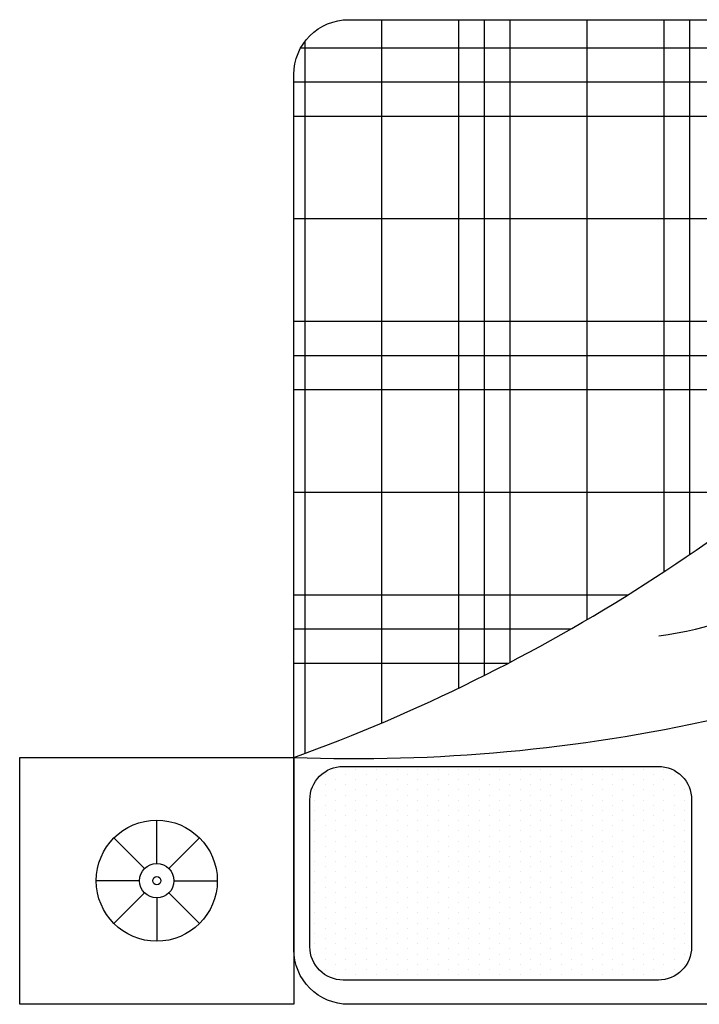
# Model space of a CAD drawing. Units: millimetres. Extents: x 2817 to 5038, y 1110 to 3565.
# Tile 20 of 21: x 4946 to 4992, y 3499 to 3565. Entities that reach past the tile are written whole.
import ezdxf

# ---------------------------------------------------------------- set-up
doc = ezdxf.new("R2010")
doc.units = ezdxf.units.MM
doc.layers.add('BLOCK', color=6, linetype='Continuous')
doc.layers.add('FURNITURE', color=219, linetype='Continuous', lineweight=18)

# ---------------------------------------------------------------- blocks, each defined once
blk = doc.blocks.new('*X7')
at = {"color": 0}
for p, q in [((276.598, 451.25), (280.51, 451.25)), ((275.455, 450.625), (280.51, 450.625)), ((274.411, 450), (280.51, 450)), ((265.51, 448.125), (267.634, 448.125)), ((271.723, 448.125), (280.51, 448.125)), ((265.51, 446.25), (268.465, 446.25)), ((269.519, 446.25), (280.51, 446.25)), ((265.51, 445.625), (268.531, 445.625)), ((268.866, 445.625), (280.51, 445.625)), ((265.51, 445), (280.51, 445)), ((265.51, 443.125), (280.51, 443.125)), ((265.51, 441.25), (280.51, 441.25)), ((265.51, 440.625), (280.51, 440.625)), ((265.634, 440), (280.386, 440))]:
    blk.add_line(p, q, dxfattribs=at)
blk = doc.blocks.new('*X8')
at = {"color": 0}
for p, q in [((280.312, 439.886), (280.312, 452.896)), ((278.906, 439.482), (278.906, 452.338)), ((277.5, 439.482), (277.5, 451.702)), ((277.031, 439.482), (277.031, 451.471)), ((276.562, 439.482), (276.562, 451.231)), ((275.156, 439.482), (275.156, 450.451)), ((265.781, 439.797), (265.781, 449.511)), ((273.75, 439.482), (273.75, 449.576)), ((266.25, 439.517), (266.25, 449.296)), ((273.281, 439.482), (273.281, 449.261)), ((272.812, 439.482), (272.812, 448.934)), ((267.656, 439.482), (267.656, 448.095)), ((271.406, 439.482), (271.406, 447.876)), ((270, 439.482), (270, 446.689)), ((269.531, 439.482), (269.531, 446.262)), ((269.062, 439.482), (269.062, 445.817))]:
    blk.add_line(p, q, dxfattribs=at)
blk = doc.blocks.new('*X9')
at = {"color": 0}
for p, q in [((273.9375, 457.03125), (273.9375, 457.03125)), ((274.3125, 457.03125), (274.3125, 457.03125)), ((274.6875, 457.03125), (274.6875, 457.03125)), ((275.0625, 457.03125), (275.0625, 457.03125)), ((275.4375, 457.03125), (275.4375, 457.03125)), ((275.8125, 457.03125), (275.8125, 457.03125)), ((276.1875, 457.03125), (276.1875, 457.03125)), ((276.5625, 457.03125), (276.5625, 457.03125)), ((276.9375, 457.03125), (276.9375, 457.03125)), ((277.3125, 457.03125), (277.3125, 457.03125)), ((277.6875, 457.03125), (277.6875, 457.03125)), ((278.0625, 457.03125), (278.0625, 457.03125)), ((278.4375, 457.03125), (278.4375, 457.03125)), ((278.8125, 457.03125), (278.8125, 457.03125)), ((279.1875, 457.03125), (279.1875, 457.03125)), ((279.5625, 457.03125), (279.5625, 457.03125)), ((273.5625, 456.84375), (273.5625, 456.84375)), ((273.75, 456.9375), (273.75, 456.9375)), ((273.9375, 456.84375), (273.9375, 456.84375)), ((274.125, 456.9375), (274.125, 456.9375)), ((274.3125, 456.84375), (274.3125, 456.84375)), ((274.5, 456.9375), (274.5, 456.9375)), ((274.6875, 456.84375), (274.6875, 456.84375)), ((274.875, 456.9375), (274.875, 456.9375)), ((275.0625, 456.84375), (275.0625, 456.84375)), ((275.25, 456.9375), (275.25, 456.9375)), ((275.4375, 456.84375), (275.4375, 456.84375)), ((275.625, 456.9375), (275.625, 456.9375)), ((275.8125, 456.84375), (275.8125, 456.84375)), ((276, 456.9375), (276, 456.9375)), ((276.1875, 456.84375), (276.1875, 456.84375)), ((276.375, 456.9375), (276.375, 456.9375)), ((276.5625, 456.84375), (276.5625, 456.84375)), ((276.75, 456.9375), (276.75, 456.9375)), ((276.9375, 456.84375), (276.9375, 456.84375)), ((277.125, 456.9375), (277.125, 456.9375)), ((277.3125, 456.84375), (277.3125, 456.84375)), ((277.5, 456.9375), (277.5, 456.9375)), ((277.6875, 456.84375), (277.6875, 456.84375)), ((277.875, 456.9375), (277.875, 456.9375)), ((278.0625, 456.84375), (278.0625, 456.84375)), ((278.25, 456.9375), (278.25, 456.9375)), ((278.4375, 456.84375), (278.4375, 456.84375)), ((278.625, 456.9375), (278.625, 456.9375)), ((278.8125, 456.84375), (278.8125, 456.84375)), ((279, 456.9375), (279, 456.9375)), ((279.1875, 456.84375), (279.1875, 456.84375)), ((279.375, 456.9375), (279.375, 456.9375)), ((279.5625, 456.84375), (279.5625, 456.84375)), ((279.75, 456.9375), (279.75, 456.9375)), ((279.9375, 456.84375), (279.9375, 456.84375)), ((273.375, 456.75), (273.375, 456.75)), ((273.75, 456.75), (273.75, 456.75)), ((274.125, 456.75), (274.125, 456.75)), ((274.5, 456.75), (274.5, 456.75)), ((274.875, 456.75), (274.875, 456.75)), ((275.25, 456.75), (275.25, 456.75)), ((275.625, 456.75), (275.625, 456.75)), ((276, 456.75), (276, 456.75)), ((276.375, 456.75), (276.375, 456.75)), ((276.75, 456.75), (276.75, 456.75)), ((277.125, 456.75), (277.125, 456.75)), ((277.5, 456.75), (277.5, 456.75)), ((277.875, 456.75), (277.875, 456.75)), ((278.25, 456.75), (278.25, 456.75)), ((278.625, 456.75), (278.625, 456.75)), ((279, 456.75), (279, 456.75)), ((279.375, 456.75), (279.375, 456.75)), ((279.75, 456.75), (279.75, 456.75)), ((280.125, 456.75), (280.125, 456.75)), ((273.375, 456.5625), (273.375, 456.5625)), ((273.5625, 456.65625), (273.5625, 456.65625)), ((273.75, 456.5625), (273.75, 456.5625)), ((273.9375, 456.65625), (273.9375, 456.65625)), ((274.125, 456.5625), (274.125, 456.5625)), ((274.3125, 456.65625), (274.3125, 456.65625)), ((274.5, 456.5625), (274.5, 456.5625)), ((274.6875, 456.65625), (274.6875, 456.65625)), ((274.875, 456.5625), (274.875, 456.5625)), ((275.0625, 456.65625), (275.0625, 456.65625)), ((275.25, 456.5625), (275.25, 456.5625)), ((275.4375, 456.65625), (275.4375, 456.65625)), ((275.625, 456.5625), (275.625, 456.5625)), ((275.8125, 456.65625), (275.8125, 456.65625)), ((276, 456.5625), (276, 456.5625)), ((276.1875, 456.65625), (276.1875, 456.65625)), ((276.375, 456.5625), (276.375, 456.5625)), ((276.5625, 456.65625), (276.5625, 456.65625)), ((276.75, 456.5625), (276.75, 456.5625)), ((276.9375, 456.65625), (276.9375, 456.65625)), ((277.125, 456.5625), (277.125, 456.5625)), ((277.3125, 456.65625), (277.3125, 456.65625)), ((277.5, 456.5625), (277.5, 456.5625)), ((277.6875, 456.65625), (277.6875, 456.65625)), ((277.875, 456.5625), (277.875, 456.5625)), ((278.0625, 456.65625), (278.0625, 456.65625)), ((278.25, 456.5625), (278.25, 456.5625)), ((278.4375, 456.65625), (278.4375, 456.65625)), ((278.625, 456.5625), (278.625, 456.5625)), ((278.8125, 456.65625), (278.8125, 456.65625)), ((279, 456.5625), (279, 456.5625)), ((279.1875, 456.65625), (279.1875, 456.65625)), ((279.375, 456.5625), (279.375, 456.5625)), ((279.5625, 456.65625), (279.5625, 456.65625)), ((279.75, 456.5625), (279.75, 456.5625)), ((279.9375, 456.65625), (279.9375, 456.65625)), ((280.125, 456.5625), (280.125, 456.5625)), ((273.375, 456.375), (273.375, 456.375)), ((273.5625, 456.46875), (273.5625, 456.46875)), ((273.75, 456.375), (273.75, 456.375)), ((273.9375, 456.46875), (273.9375, 456.46875)), ((274.125, 456.375), (274.125, 456.375)), ((274.3125, 456.46875), (274.3125, 456.46875)), ((274.5, 456.375), (274.5, 456.375)), ((274.6875, 456.46875), (274.6875, 456.46875)), ((274.875, 456.375), (274.875, 456.375)), ((275.0625, 456.46875), (275.0625, 456.46875)), ((275.25, 456.375), (275.25, 456.375)), ((275.4375, 456.46875), (275.4375, 456.46875)), ((275.625, 456.375), (275.625, 456.375)), ((275.8125, 456.46875), (275.8125, 456.46875)), ((276, 456.375), (276, 456.375)), ((276.1875, 456.46875), (276.1875, 456.46875)), ((276.375, 456.375), (276.375, 456.375)), ((276.5625, 456.46875), (276.5625, 456.46875)), ((276.75, 456.375), (276.75, 456.375)), ((276.9375, 456.46875), (276.9375, 456.46875)), ((277.125, 456.375), (277.125, 456.375)), ((277.3125, 456.46875), (277.3125, 456.46875)), ((277.5, 456.375), (277.5, 456.375)), ((277.6875, 456.46875), (277.6875, 456.46875)), ((277.875, 456.375), (277.875, 456.375)), ((278.0625, 456.46875), (278.0625, 456.46875)), ((278.25, 456.375), (278.25, 456.375)), ((278.4375, 456.46875), (278.4375, 456.46875)), ((278.625, 456.375), (278.625, 456.375)), ((278.8125, 456.46875), (278.8125, 456.46875)), ((279, 456.375), (279, 456.375)), ((279.1875, 456.46875), (279.1875, 456.46875)), ((279.375, 456.375), (279.375, 456.375)), ((279.5625, 456.46875), (279.5625, 456.46875)), ((279.75, 456.375), (279.75, 456.375)), ((279.9375, 456.46875), (279.9375, 456.46875)), ((280.125, 456.375), (280.125, 456.375)), ((273.375, 456.1875), (273.375, 456.1875)), ((273.5625, 456.28125), (273.5625, 456.28125)), ((273.75, 456.1875), (273.75, 456.1875)), ((273.9375, 456.28125), (273.9375, 456.28125)), ((274.125, 456.1875), (274.125, 456.1875)), ((274.3125, 456.28125), (274.3125, 456.28125)), ((274.5, 456.1875), (274.5, 456.1875)), ((274.6875, 456.28125), (274.6875, 456.28125)), ((274.875, 456.1875), (274.875, 456.1875)), ((275.0625, 456.28125), (275.0625, 456.28125)), ((275.25, 456.1875), (275.25, 456.1875)), ((275.4375, 456.28125), (275.4375, 456.28125)), ((275.625, 456.1875), (275.625, 456.1875)), ((275.8125, 456.28125), (275.8125, 456.28125)), ((276, 456.1875), (276, 456.1875)), ((276.1875, 456.28125), (276.1875, 456.28125)), ((276.375, 456.1875), (276.375, 456.1875)), ((276.5625, 456.28125), (276.5625, 456.28125)), ((276.75, 456.1875), (276.75, 456.1875)), ((276.9375, 456.28125), (276.9375, 456.28125)), ((277.125, 456.1875), (277.125, 456.1875)), ((277.3125, 456.28125), (277.3125, 456.28125)), ((277.5, 456.1875), (277.5, 456.1875)), ((277.6875, 456.28125), (277.6875, 456.28125)), ((277.875, 456.1875), (277.875, 456.1875)), ((278.0625, 456.28125), (278.0625, 456.28125)), ((278.25, 456.1875), (278.25, 456.1875)), ((278.4375, 456.28125), (278.4375, 456.28125)), ((278.625, 456.1875), (278.625, 456.1875)), ((278.8125, 456.28125), (278.8125, 456.28125)), ((279, 456.1875), (279, 456.1875)), ((279.1875, 456.28125), (279.1875, 456.28125)), ((279.375, 456.1875), (279.375, 456.1875)), ((279.5625, 456.28125), (279.5625, 456.28125)), ((279.75, 456.1875), (279.75, 456.1875)), ((279.9375, 456.28125), (279.9375, 456.28125)), ((280.125, 456.1875), (280.125, 456.1875)), ((273.375, 456), (273.375, 456)), ((273.5625, 456.09375), (273.5625, 456.09375)), ((273.75, 456), (273.75, 456)), ((273.9375, 456.09375), (273.9375, 456.09375)), ((274.125, 456), (274.125, 456)), ((274.3125, 456.09375), (274.3125, 456.09375)), ((274.5, 456), (274.5, 456)), ((274.6875, 456.09375), (274.6875, 456.09375)), ((274.875, 456), (274.875, 456)), ((275.0625, 456.09375), (275.0625, 456.09375)), ((275.25, 456), (275.25, 456)), ((275.4375, 456.09375), (275.4375, 456.09375)), ((275.625, 456), (275.625, 456)), ((275.8125, 456.09375), (275.8125, 456.09375)), ((276, 456), (276, 456)), ((276.1875, 456.09375), (276.1875, 456.09375)), ((276.375, 456), (276.375, 456)), ((276.5625, 456.09375), (276.5625, 456.09375)), ((276.75, 456), (276.75, 456)), ((276.9375, 456.09375), (276.9375, 456.09375)), ((277.125, 456), (277.125, 456)), ((277.3125, 456.09375), (277.3125, 456.09375)), ((277.5, 456), (277.5, 456)), ((277.6875, 456.09375), (277.6875, 456.09375)), ((277.875, 456), (277.875, 456)), ((278.0625, 456.09375), (278.0625, 456.09375)), ((278.25, 456), (278.25, 456)), ((278.4375, 456.09375), (278.4375, 456.09375)), ((278.625, 456), (278.625, 456)), ((278.8125, 456.09375), (278.8125, 456.09375)), ((279, 456), (279, 456)), ((279.1875, 456.09375), (279.1875, 456.09375)), ((279.375, 456), (279.375, 456)), ((279.5625, 456.09375), (279.5625, 456.09375)), ((279.75, 456), (279.75, 456)), ((279.9375, 456.09375), (279.9375, 456.09375)), ((280.125, 456), (280.125, 456)), ((273.375, 455.8125), (273.375, 455.8125)), ((273.5625, 455.90625), (273.5625, 455.90625)), ((273.75, 455.8125), (273.75, 455.8125)), ((273.9375, 455.90625), (273.9375, 455.90625)), ((274.125, 455.8125), (274.125, 455.8125)), ((274.3125, 455.90625), (274.3125, 455.90625)), ((274.5, 455.8125), (274.5, 455.8125)), ((274.6875, 455.90625), (274.6875, 455.90625)), ((274.875, 455.8125), (274.875, 455.8125)), ((275.0625, 455.90625), (275.0625, 455.90625)), ((275.25, 455.8125), (275.25, 455.8125)), ((275.4375, 455.90625), (275.4375, 455.90625)), ((275.625, 455.8125), (275.625, 455.8125)), ((275.8125, 455.90625), (275.8125, 455.90625)), ((276, 455.8125), (276, 455.8125)), ((276.1875, 455.90625), (276.1875, 455.90625)), ((276.375, 455.8125), (276.375, 455.8125)), ((276.5625, 455.90625), (276.5625, 455.90625)), ((276.75, 455.8125), (276.75, 455.8125)), ((276.9375, 455.90625), (276.9375, 455.90625)), ((277.125, 455.8125), (277.125, 455.8125)), ((277.3125, 455.90625), (277.3125, 455.90625)), ((277.5, 455.8125), (277.5, 455.8125)), ((277.6875, 455.90625), (277.6875, 455.90625)), ((277.875, 455.8125), (277.875, 455.8125)), ((278.0625, 455.90625), (278.0625, 455.90625)), ((278.25, 455.8125), (278.25, 455.8125)), ((278.4375, 455.90625), (278.4375, 455.90625)), ((278.625, 455.8125), (278.625, 455.8125)), ((278.8125, 455.90625), (278.8125, 455.90625)), ((279, 455.8125), (279, 455.8125)), ((279.1875, 455.90625), (279.1875, 455.90625)), ((279.375, 455.8125), (279.375, 455.8125)), ((279.5625, 455.90625), (279.5625, 455.90625)), ((279.75, 455.8125), (279.75, 455.8125)), ((279.9375, 455.90625), (279.9375, 455.90625)), ((280.125, 455.8125), (280.125, 455.8125)), ((273.375, 455.625), (273.375, 455.625)), ((273.5625, 455.71875), (273.5625, 455.71875)), ((273.75, 455.625), (273.75, 455.625)), ((273.9375, 455.71875), (273.9375, 455.71875)), ((274.125, 455.625), (274.125, 455.625)), ((274.3125, 455.71875), (274.3125, 455.71875)), ((274.5, 455.625), (274.5, 455.625)), ((274.6875, 455.71875), (274.6875, 455.71875)), ((274.875, 455.625), (274.875, 455.625)), ((275.0625, 455.71875), (275.0625, 455.71875)), ((275.25, 455.625), (275.25, 455.625)), ((275.4375, 455.71875), (275.4375, 455.71875)), ((275.625, 455.625), (275.625, 455.625)), ((275.8125, 455.71875), (275.8125, 455.71875)), ((276, 455.625), (276, 455.625)), ((276.1875, 455.71875), (276.1875, 455.71875)), ((276.375, 455.625), (276.375, 455.625)), ((276.5625, 455.71875), (276.5625, 455.71875)), ((276.75, 455.625), (276.75, 455.625)), ((276.9375, 455.71875), (276.9375, 455.71875)), ((277.125, 455.625), (277.125, 455.625)), ((277.3125, 455.71875), (277.3125, 455.71875)), ((277.5, 455.625), (277.5, 455.625)), ((277.6875, 455.71875), (277.6875, 455.71875)), ((277.875, 455.625), (277.875, 455.625)), ((278.0625, 455.71875), (278.0625, 455.71875)), ((278.25, 455.625), (278.25, 455.625)), ((278.4375, 455.71875), (278.4375, 455.71875)), ((278.625, 455.625), (278.625, 455.625)), ((278.8125, 455.71875), (278.8125, 455.71875)), ((279, 455.625), (279, 455.625)), ((279.1875, 455.71875), (279.1875, 455.71875)), ((279.375, 455.625), (279.375, 455.625)), ((279.5625, 455.71875), (279.5625, 455.71875)), ((279.75, 455.625), (279.75, 455.625)), ((279.9375, 455.71875), (279.9375, 455.71875)), ((280.125, 455.625), (280.125, 455.625)), ((273.375, 455.4375), (273.375, 455.4375)), ((273.5625, 455.53125), (273.5625, 455.53125)), ((273.75, 455.4375), (273.75, 455.4375)), ((273.9375, 455.53125), (273.9375, 455.53125)), ((274.125, 455.4375), (274.125, 455.4375)), ((274.3125, 455.53125), (274.3125, 455.53125)), ((274.5, 455.4375), (274.5, 455.4375)), ((274.6875, 455.53125), (274.6875, 455.53125)), ((274.875, 455.4375), (274.875, 455.4375)), ((275.0625, 455.53125), (275.0625, 455.53125)), ((275.25, 455.4375), (275.25, 455.4375)), ((275.4375, 455.53125), (275.4375, 455.53125)), ((275.625, 455.4375), (275.625, 455.4375)), ((275.8125, 455.53125), (275.8125, 455.53125)), ((276, 455.4375), (276, 455.4375)), ((276.1875, 455.53125), (276.1875, 455.53125)), ((276.375, 455.4375), (276.375, 455.4375)), ((276.5625, 455.53125), (276.5625, 455.53125)), ((276.75, 455.4375), (276.75, 455.4375)), ((276.9375, 455.53125), (276.9375, 455.53125)), ((277.125, 455.4375), (277.125, 455.4375)), ((277.3125, 455.53125), (277.3125, 455.53125)), ((277.5, 455.4375), (277.5, 455.4375)), ((277.6875, 455.53125), (277.6875, 455.53125)), ((277.875, 455.4375), (277.875, 455.4375)), ((278.0625, 455.53125), (278.0625, 455.53125)), ((278.25, 455.4375), (278.25, 455.4375)), ((278.4375, 455.53125), (278.4375, 455.53125)), ((278.625, 455.4375), (278.625, 455.4375)), ((278.8125, 455.53125), (278.8125, 455.53125)), ((279, 455.4375), (279, 455.4375)), ((279.1875, 455.53125), (279.1875, 455.53125)), ((279.375, 455.4375), (279.375, 455.4375)), ((279.5625, 455.53125), (279.5625, 455.53125)), ((279.75, 455.4375), (279.75, 455.4375)), ((279.9375, 455.53125), (279.9375, 455.53125)), ((280.125, 455.4375), (280.125, 455.4375)), ((273.375, 455.25), (273.375, 455.25)), ((273.5625, 455.34375), (273.5625, 455.34375)), ((273.75, 455.25), (273.75, 455.25)), ((273.9375, 455.34375), (273.9375, 455.34375)), ((274.125, 455.25), (274.125, 455.25)), ((274.3125, 455.34375), (274.3125, 455.34375)), ((274.5, 455.25), (274.5, 455.25)), ((274.6875, 455.34375), (274.6875, 455.34375)), ((274.875, 455.25), (274.875, 455.25)), ((275.0625, 455.34375), (275.0625, 455.34375)), ((275.25, 455.25), (275.25, 455.25)), ((275.4375, 455.34375), (275.4375, 455.34375)), ((275.625, 455.25), (275.625, 455.25)), ((275.8125, 455.34375), (275.8125, 455.34375)), ((276, 455.25), (276, 455.25)), ((276.1875, 455.34375), (276.1875, 455.34375)), ((276.375, 455.25), (276.375, 455.25)), ((276.5625, 455.34375), (276.5625, 455.34375)), ((276.75, 455.25), (276.75, 455.25)), ((276.9375, 455.34375), (276.9375, 455.34375)), ((277.125, 455.25), (277.125, 455.25)), ((277.3125, 455.34375), (277.3125, 455.34375)), ((277.5, 455.25), (277.5, 455.25)), ((277.6875, 455.34375), (277.6875, 455.34375)), ((277.875, 455.25), (277.875, 455.25)), ((278.0625, 455.34375), (278.0625, 455.34375)), ((278.25, 455.25), (278.25, 455.25)), ((278.4375, 455.34375), (278.4375, 455.34375)), ((278.625, 455.25), (278.625, 455.25)), ((278.8125, 455.34375), (278.8125, 455.34375)), ((279, 455.25), (279, 455.25)), ((279.1875, 455.34375), (279.1875, 455.34375)), ((279.375, 455.25), (279.375, 455.25)), ((279.5625, 455.34375), (279.5625, 455.34375)), ((279.75, 455.25), (279.75, 455.25)), ((279.9375, 455.34375), (279.9375, 455.34375)), ((280.125, 455.25), (280.125, 455.25)), ((273.375, 455.0625), (273.375, 455.0625)), ((273.5625, 455.15625), (273.5625, 455.15625)), ((273.75, 455.0625), (273.75, 455.0625)), ((273.9375, 455.15625), (273.9375, 455.15625)), ((274.125, 455.0625), (274.125, 455.0625)), ((274.3125, 455.15625), (274.3125, 455.15625)), ((274.5, 455.0625), (274.5, 455.0625)), ((274.6875, 455.15625), (274.6875, 455.15625)), ((274.875, 455.0625), (274.875, 455.0625)), ((275.0625, 455.15625), (275.0625, 455.15625)), ((275.25, 455.0625), (275.25, 455.0625)), ((275.4375, 455.15625), (275.4375, 455.15625)), ((275.625, 455.0625), (275.625, 455.0625)), ((275.8125, 455.15625), (275.8125, 455.15625)), ((276, 455.0625), (276, 455.0625)), ((276.1875, 455.15625), (276.1875, 455.15625)), ((276.375, 455.0625), (276.375, 455.0625)), ((276.5625, 455.15625), (276.5625, 455.15625)), ((276.75, 455.0625), (276.75, 455.0625)), ((276.9375, 455.15625), (276.9375, 455.15625)), ((277.125, 455.0625), (277.125, 455.0625)), ((277.3125, 455.15625), (277.3125, 455.15625)), ((277.5, 455.0625), (277.5, 455.0625)), ((277.6875, 455.15625), (277.6875, 455.15625)), ((277.875, 455.0625), (277.875, 455.0625)), ((278.0625, 455.15625), (278.0625, 455.15625)), ((278.25, 455.0625), (278.25, 455.0625)), ((278.4375, 455.15625), (278.4375, 455.15625)), ((278.625, 455.0625), (278.625, 455.0625)), ((278.8125, 455.15625), (278.8125, 455.15625)), ((279, 455.0625), (279, 455.0625)), ((279.1875, 455.15625), (279.1875, 455.15625)), ((279.375, 455.0625), (279.375, 455.0625)), ((279.5625, 455.15625), (279.5625, 455.15625)), ((279.75, 455.0625), (279.75, 455.0625)), ((279.9375, 455.15625), (279.9375, 455.15625)), ((280.125, 455.0625), (280.125, 455.0625)), ((273.375, 454.875), (273.375, 454.875)), ((273.5625, 454.96875), (273.5625, 454.96875)), ((273.75, 454.875), (273.75, 454.875)), ((273.9375, 454.96875), (273.9375, 454.96875)), ((274.125, 454.875), (274.125, 454.875)), ((274.3125, 454.96875), (274.3125, 454.96875)), ((274.5, 454.875), (274.5, 454.875)), ((274.6875, 454.96875), (274.6875, 454.96875)), ((274.875, 454.875), (274.875, 454.875)), ((275.0625, 454.96875), (275.0625, 454.96875)), ((275.25, 454.875), (275.25, 454.875)), ((275.4375, 454.96875), (275.4375, 454.96875)), ((275.625, 454.875), (275.625, 454.875)), ((275.8125, 454.96875), (275.8125, 454.96875)), ((276, 454.875), (276, 454.875)), ((276.1875, 454.96875), (276.1875, 454.96875)), ((276.375, 454.875), (276.375, 454.875)), ((276.5625, 454.96875), (276.5625, 454.96875)), ((276.75, 454.875), (276.75, 454.875)), ((276.9375, 454.96875), (276.9375, 454.96875)), ((277.125, 454.875), (277.125, 454.875)), ((277.3125, 454.96875), (277.3125, 454.96875)), ((277.5, 454.875), (277.5, 454.875)), ((277.6875, 454.96875), (277.6875, 454.96875)), ((277.875, 454.875), (277.875, 454.875)), ((278.0625, 454.96875), (278.0625, 454.96875)), ((278.25, 454.875), (278.25, 454.875)), ((278.4375, 454.96875), (278.4375, 454.96875)), ((278.625, 454.875), (278.625, 454.875)), ((278.8125, 454.96875), (278.8125, 454.96875)), ((279, 454.875), (279, 454.875)), ((279.1875, 454.96875), (279.1875, 454.96875)), ((279.375, 454.875), (279.375, 454.875)), ((279.5625, 454.96875), (279.5625, 454.96875)), ((279.75, 454.875), (279.75, 454.875)), ((279.9375, 454.96875), (279.9375, 454.96875)), ((280.125, 454.875), (280.125, 454.875)), ((273.375, 454.6875), (273.375, 454.6875)), ((273.5625, 454.78125), (273.5625, 454.78125)), ((273.75, 454.6875), (273.75, 454.6875)), ((273.9375, 454.78125), (273.9375, 454.78125)), ((274.125, 454.6875), (274.125, 454.6875)), ((274.3125, 454.78125), (274.3125, 454.78125)), ((274.5, 454.6875), (274.5, 454.6875)), ((274.6875, 454.78125), (274.6875, 454.78125)), ((274.875, 454.6875), (274.875, 454.6875)), ((275.0625, 454.78125), (275.0625, 454.78125)), ((275.25, 454.6875), (275.25, 454.6875)), ((275.4375, 454.78125), (275.4375, 454.78125)), ((275.625, 454.6875), (275.625, 454.6875)), ((275.8125, 454.78125), (275.8125, 454.78125)), ((276, 454.6875), (276, 454.6875)), ((276.1875, 454.78125), (276.1875, 454.78125)), ((276.375, 454.6875), (276.375, 454.6875)), ((276.5625, 454.78125), (276.5625, 454.78125)), ((276.75, 454.6875), (276.75, 454.6875)), ((276.9375, 454.78125), (276.9375, 454.78125)), ((277.125, 454.6875), (277.125, 454.6875)), ((277.3125, 454.78125), (277.3125, 454.78125)), ((277.5, 454.6875), (277.5, 454.6875)), ((277.6875, 454.78125), (277.6875, 454.78125)), ((277.875, 454.6875), (277.875, 454.6875)), ((278.0625, 454.78125), (278.0625, 454.78125)), ((278.25, 454.6875), (278.25, 454.6875)), ((278.4375, 454.78125), (278.4375, 454.78125)), ((278.625, 454.6875), (278.625, 454.6875)), ((278.8125, 454.78125), (278.8125, 454.78125)), ((279, 454.6875), (279, 454.6875)), ((279.1875, 454.78125), (279.1875, 454.78125)), ((279.375, 454.6875), (279.375, 454.6875)), ((279.5625, 454.78125), (279.5625, 454.78125)), ((279.75, 454.6875), (279.75, 454.6875)), ((279.9375, 454.78125), (279.9375, 454.78125)), ((280.125, 454.6875), (280.125, 454.6875)), ((273.5625, 454.59375), (273.5625, 454.59375)), ((273.9375, 454.59375), (273.9375, 454.59375)), ((274.3125, 454.59375), (274.3125, 454.59375)), ((274.6875, 454.59375), (274.6875, 454.59375)), ((275.0625, 454.59375), (275.0625, 454.59375)), ((275.4375, 454.59375), (275.4375, 454.59375)), ((275.8125, 454.59375), (275.8125, 454.59375)), ((276.1875, 454.59375), (276.1875, 454.59375)), ((276.5625, 454.59375), (276.5625, 454.59375)), ((276.9375, 454.59375), (276.9375, 454.59375)), ((277.3125, 454.59375), (277.3125, 454.59375)), ((277.6875, 454.59375), (277.6875, 454.59375)), ((278.0625, 454.59375), (278.0625, 454.59375)), ((278.4375, 454.59375), (278.4375, 454.59375)), ((278.8125, 454.59375), (278.8125, 454.59375)), ((279.1875, 454.59375), (279.1875, 454.59375)), ((279.5625, 454.59375), (279.5625, 454.59375)), ((279.9375, 454.59375), (279.9375, 454.59375)), ((273.375, 454.5), (273.375, 454.5)), ((273.5625, 454.40625), (273.5625, 454.40625)), ((273.75, 454.5), (273.75, 454.5)), ((273.9375, 454.40625), (273.9375, 454.40625)), ((274.125, 454.5), (274.125, 454.5)), ((274.3125, 454.40625), (274.3125, 454.40625)), ((274.5, 454.5), (274.5, 454.5)), ((274.6875, 454.40625), (274.6875, 454.40625)), ((274.875, 454.5), (274.875, 454.5)), ((275.0625, 454.40625), (275.0625, 454.40625)), ((275.25, 454.5), (275.25, 454.5)), ((275.4375, 454.40625), (275.4375, 454.40625)), ((275.625, 454.5), (275.625, 454.5)), ((275.8125, 454.40625), (275.8125, 454.40625)), ((276, 454.5), (276, 454.5)), ((276.1875, 454.40625), (276.1875, 454.40625)), ((276.375, 454.5), (276.375, 454.5)), ((276.5625, 454.40625), (276.5625, 454.40625)), ((276.75, 454.5), (276.75, 454.5)), ((276.9375, 454.40625), (276.9375, 454.40625)), ((277.125, 454.5), (277.125, 454.5)), ((277.3125, 454.40625), (277.3125, 454.40625)), ((277.5, 454.5), (277.5, 454.5)), ((277.6875, 454.40625), (277.6875, 454.40625)), ((277.875, 454.5), (277.875, 454.5)), ((278.0625, 454.40625), (278.0625, 454.40625)), ((278.25, 454.5), (278.25, 454.5)), ((278.4375, 454.40625), (278.4375, 454.40625)), ((278.625, 454.5), (278.625, 454.5)), ((278.8125, 454.40625), (278.8125, 454.40625)), ((279, 454.5), (279, 454.5)), ((279.1875, 454.40625), (279.1875, 454.40625)), ((279.375, 454.5), (279.375, 454.5)), ((279.5625, 454.40625), (279.5625, 454.40625)), ((279.75, 454.5), (279.75, 454.5)), ((279.9375, 454.40625), (279.9375, 454.40625)), ((280.125, 454.5), (280.125, 454.5)), ((273.375, 454.3125), (273.375, 454.3125)), ((273.5625, 454.21875), (273.5625, 454.21875)), ((273.75, 454.3125), (273.75, 454.3125)), ((273.9375, 454.21875), (273.9375, 454.21875)), ((274.125, 454.3125), (274.125, 454.3125)), ((274.3125, 454.21875), (274.3125, 454.21875)), ((274.5, 454.3125), (274.5, 454.3125)), ((274.6875, 454.21875), (274.6875, 454.21875)), ((274.875, 454.3125), (274.875, 454.3125)), ((275.0625, 454.21875), (275.0625, 454.21875)), ((275.25, 454.3125), (275.25, 454.3125)), ((275.4375, 454.21875), (275.4375, 454.21875)), ((275.625, 454.3125), (275.625, 454.3125)), ((275.8125, 454.21875), (275.8125, 454.21875)), ((276, 454.3125), (276, 454.3125)), ((276.1875, 454.21875), (276.1875, 454.21875)), ((276.375, 454.3125), (276.375, 454.3125)), ((276.5625, 454.21875), (276.5625, 454.21875)), ((276.75, 454.3125), (276.75, 454.3125)), ((276.9375, 454.21875), (276.9375, 454.21875)), ((277.125, 454.3125), (277.125, 454.3125)), ((277.3125, 454.21875), (277.3125, 454.21875)), ((277.5, 454.3125), (277.5, 454.3125)), ((277.6875, 454.21875), (277.6875, 454.21875)), ((277.875, 454.3125), (277.875, 454.3125)), ((278.0625, 454.21875), (278.0625, 454.21875)), ((278.25, 454.3125), (278.25, 454.3125)), ((278.4375, 454.21875), (278.4375, 454.21875)), ((278.625, 454.3125), (278.625, 454.3125)), ((278.8125, 454.21875), (278.8125, 454.21875)), ((279, 454.3125), (279, 454.3125)), ((279.1875, 454.21875), (279.1875, 454.21875)), ((279.375, 454.3125), (279.375, 454.3125)), ((279.5625, 454.21875), (279.5625, 454.21875)), ((279.75, 454.3125), (279.75, 454.3125)), ((279.9375, 454.21875), (279.9375, 454.21875)), ((280.125, 454.3125), (280.125, 454.3125)), ((273.375, 454.125), (273.375, 454.125)), ((273.5625, 454.03125), (273.5625, 454.03125)), ((273.75, 454.125), (273.75, 454.125)), ((273.9375, 454.03125), (273.9375, 454.03125)), ((274.125, 454.125), (274.125, 454.125)), ((274.3125, 454.03125), (274.3125, 454.03125)), ((274.5, 454.125), (274.5, 454.125)), ((274.6875, 454.03125), (274.6875, 454.03125)), ((274.875, 454.125), (274.875, 454.125)), ((275.0625, 454.03125), (275.0625, 454.03125)), ((275.25, 454.125), (275.25, 454.125)), ((275.4375, 454.03125), (275.4375, 454.03125)), ((275.625, 454.125), (275.625, 454.125)), ((275.8125, 454.03125), (275.8125, 454.03125)), ((276, 454.125), (276, 454.125)), ((276.1875, 454.03125), (276.1875, 454.03125)), ((276.375, 454.125), (276.375, 454.125)), ((276.5625, 454.03125), (276.5625, 454.03125)), ((276.75, 454.125), (276.75, 454.125)), ((276.9375, 454.03125), (276.9375, 454.03125)), ((277.125, 454.125), (277.125, 454.125)), ((277.3125, 454.03125), (277.3125, 454.03125)), ((277.5, 454.125), (277.5, 454.125)), ((277.6875, 454.03125), (277.6875, 454.03125)), ((277.875, 454.125), (277.875, 454.125)), ((278.0625, 454.03125), (278.0625, 454.03125)), ((278.25, 454.125), (278.25, 454.125)), ((278.4375, 454.03125), (278.4375, 454.03125)), ((278.625, 454.125), (278.625, 454.125)), ((278.8125, 454.03125), (278.8125, 454.03125)), ((279, 454.125), (279, 454.125)), ((279.1875, 454.03125), (279.1875, 454.03125)), ((279.375, 454.125), (279.375, 454.125)), ((279.5625, 454.03125), (279.5625, 454.03125)), ((279.75, 454.125), (279.75, 454.125)), ((279.9375, 454.03125), (279.9375, 454.03125)), ((280.125, 454.125), (280.125, 454.125)), ((273.375, 453.9375), (273.375, 453.9375)), ((273.5625, 453.84375), (273.5625, 453.84375)), ((273.75, 453.9375), (273.75, 453.9375)), ((273.9375, 453.84375), (273.9375, 453.84375)), ((274.125, 453.9375), (274.125, 453.9375)), ((274.3125, 453.84375), (274.3125, 453.84375)), ((274.5, 453.9375), (274.5, 453.9375)), ((274.6875, 453.84375), (274.6875, 453.84375)), ((274.875, 453.9375), (274.875, 453.9375)), ((275.0625, 453.84375), (275.0625, 453.84375)), ((275.25, 453.9375), (275.25, 453.9375)), ((275.4375, 453.84375), (275.4375, 453.84375)), ((275.625, 453.9375), (275.625, 453.9375)), ((275.8125, 453.84375), (275.8125, 453.84375)), ((276, 453.9375), (276, 453.9375)), ((276.1875, 453.84375), (276.1875, 453.84375)), ((276.375, 453.9375), (276.375, 453.9375)), ((276.5625, 453.84375), (276.5625, 453.84375)), ((276.75, 453.9375), (276.75, 453.9375)), ((276.9375, 453.84375), (276.9375, 453.84375)), ((277.125, 453.9375), (277.125, 453.9375)), ((277.3125, 453.84375), (277.3125, 453.84375)), ((277.5, 453.9375), (277.5, 453.9375)), ((277.6875, 453.84375), (277.6875, 453.84375)), ((277.875, 453.9375), (277.875, 453.9375)), ((278.0625, 453.84375), (278.0625, 453.84375)), ((278.25, 453.9375), (278.25, 453.9375)), ((278.4375, 453.84375), (278.4375, 453.84375)), ((278.625, 453.9375), (278.625, 453.9375)), ((278.8125, 453.84375), (278.8125, 453.84375)), ((279, 453.9375), (279, 453.9375)), ((279.1875, 453.84375), (279.1875, 453.84375)), ((279.375, 453.9375), (279.375, 453.9375)), ((279.5625, 453.84375), (279.5625, 453.84375)), ((279.75, 453.9375), (279.75, 453.9375)), ((279.9375, 453.84375), (279.9375, 453.84375)), ((280.125, 453.9375), (280.125, 453.9375)), ((273.375, 453.75), (273.375, 453.75)), ((273.5625, 453.65625), (273.5625, 453.65625)), ((273.75, 453.75), (273.75, 453.75)), ((273.9375, 453.65625), (273.9375, 453.65625)), ((274.125, 453.75), (274.125, 453.75)), ((274.3125, 453.65625), (274.3125, 453.65625)), ((274.5, 453.75), (274.5, 453.75)), ((274.6875, 453.65625), (274.6875, 453.65625)), ((274.875, 453.75), (274.875, 453.75)), ((275.0625, 453.65625), (275.0625, 453.65625)), ((275.25, 453.75), (275.25, 453.75)), ((275.4375, 453.65625), (275.4375, 453.65625)), ((275.625, 453.75), (275.625, 453.75)), ((275.8125, 453.65625), (275.8125, 453.65625)), ((276, 453.75), (276, 453.75)), ((276.1875, 453.65625), (276.1875, 453.65625)), ((276.375, 453.75), (276.375, 453.75)), ((276.5625, 453.65625), (276.5625, 453.65625)), ((276.75, 453.75), (276.75, 453.75)), ((276.9375, 453.65625), (276.9375, 453.65625)), ((277.125, 453.75), (277.125, 453.75)), ((277.3125, 453.65625), (277.3125, 453.65625)), ((277.5, 453.75), (277.5, 453.75)), ((277.6875, 453.65625), (277.6875, 453.65625)), ((277.875, 453.75), (277.875, 453.75)), ((278.0625, 453.65625), (278.0625, 453.65625)), ((278.25, 453.75), (278.25, 453.75)), ((278.4375, 453.65625), (278.4375, 453.65625)), ((278.625, 453.75), (278.625, 453.75)), ((278.8125, 453.65625), (278.8125, 453.65625)), ((279, 453.75), (279, 453.75)), ((279.1875, 453.65625), (279.1875, 453.65625)), ((279.375, 453.75), (279.375, 453.75)), ((279.5625, 453.65625), (279.5625, 453.65625)), ((279.75, 453.75), (279.75, 453.75)), ((279.9375, 453.65625), (279.9375, 453.65625)), ((280.125, 453.75), (280.125, 453.75)), ((273.375, 453.5625), (273.375, 453.5625)), ((273.5625, 453.46875), (273.5625, 453.46875)), ((273.75, 453.5625), (273.75, 453.5625)), ((273.9375, 453.46875), (273.9375, 453.46875)), ((274.125, 453.5625), (274.125, 453.5625)), ((274.3125, 453.46875), (274.3125, 453.46875)), ((274.5, 453.5625), (274.5, 453.5625)), ((274.6875, 453.46875), (274.6875, 453.46875)), ((274.875, 453.5625), (274.875, 453.5625)), ((275.0625, 453.46875), (275.0625, 453.46875)), ((275.25, 453.5625), (275.25, 453.5625)), ((275.4375, 453.46875), (275.4375, 453.46875)), ((275.625, 453.5625), (275.625, 453.5625)), ((275.8125, 453.46875), (275.8125, 453.46875)), ((276, 453.5625), (276, 453.5625)), ((276.1875, 453.46875), (276.1875, 453.46875)), ((276.375, 453.5625), (276.375, 453.5625)), ((276.5625, 453.46875), (276.5625, 453.46875)), ((276.75, 453.5625), (276.75, 453.5625)), ((276.9375, 453.46875), (276.9375, 453.46875)), ((277.125, 453.5625), (277.125, 453.5625)), ((277.3125, 453.46875), (277.3125, 453.46875)), ((277.5, 453.5625), (277.5, 453.5625)), ((277.6875, 453.46875), (277.6875, 453.46875)), ((277.875, 453.5625), (277.875, 453.5625)), ((278.0625, 453.46875), (278.0625, 453.46875)), ((278.25, 453.5625), (278.25, 453.5625)), ((278.4375, 453.46875), (278.4375, 453.46875)), ((278.625, 453.5625), (278.625, 453.5625)), ((278.8125, 453.46875), (278.8125, 453.46875)), ((279, 453.5625), (279, 453.5625)), ((279.1875, 453.46875), (279.1875, 453.46875)), ((279.375, 453.5625), (279.375, 453.5625)), ((279.5625, 453.46875), (279.5625, 453.46875)), ((279.75, 453.5625), (279.75, 453.5625)), ((279.9375, 453.46875), (279.9375, 453.46875)), ((280.125, 453.5625), (280.125, 453.5625)), ((273.375, 453.375), (273.375, 453.375)), ((273.5625, 453.28125), (273.5625, 453.28125)), ((273.75, 453.375), (273.75, 453.375)), ((273.9375, 453.28125), (273.9375, 453.28125)), ((274.125, 453.375), (274.125, 453.375)), ((274.3125, 453.28125), (274.3125, 453.28125)), ((274.5, 453.375), (274.5, 453.375)), ((274.6875, 453.28125), (274.6875, 453.28125)), ((274.875, 453.375), (274.875, 453.375)), ((275.0625, 453.28125), (275.0625, 453.28125)), ((275.25, 453.375), (275.25, 453.375)), ((275.4375, 453.28125), (275.4375, 453.28125)), ((275.625, 453.375), (275.625, 453.375)), ((275.8125, 453.28125), (275.8125, 453.28125)), ((276, 453.375), (276, 453.375)), ((276.1875, 453.28125), (276.1875, 453.28125)), ((276.375, 453.375), (276.375, 453.375)), ((276.5625, 453.28125), (276.5625, 453.28125)), ((276.75, 453.375), (276.75, 453.375)), ((276.9375, 453.28125), (276.9375, 453.28125)), ((277.125, 453.375), (277.125, 453.375)), ((277.3125, 453.28125), (277.3125, 453.28125)), ((277.5, 453.375), (277.5, 453.375)), ((277.6875, 453.28125), (277.6875, 453.28125)), ((277.875, 453.375), (277.875, 453.375)), ((278.0625, 453.28125), (278.0625, 453.28125)), ((278.25, 453.375), (278.25, 453.375)), ((278.4375, 453.28125), (278.4375, 453.28125)), ((278.625, 453.375), (278.625, 453.375)), ((278.8125, 453.28125), (278.8125, 453.28125)), ((279, 453.375), (279, 453.375)), ((279.1875, 453.28125), (279.1875, 453.28125)), ((279.375, 453.375), (279.375, 453.375)), ((279.5625, 453.28125), (279.5625, 453.28125)), ((279.75, 453.375), (279.75, 453.375)), ((279.9375, 453.28125), (279.9375, 453.28125)), ((273.75, 453.1875), (273.75, 453.1875)), ((274.125, 453.1875), (274.125, 453.1875)), ((274.5, 453.1875), (274.5, 453.1875)), ((274.875, 453.1875), (274.875, 453.1875)), ((275.25, 453.1875), (275.25, 453.1875)), ((275.625, 453.1875), (275.625, 453.1875)), ((276, 453.1875), (276, 453.1875)), ((276.375, 453.1875), (276.375, 453.1875)), ((276.75, 453.1875), (276.75, 453.1875)), ((277.125, 453.1875), (277.125, 453.1875)), ((277.5, 453.1875), (277.5, 453.1875)), ((277.875, 453.1875), (277.875, 453.1875)), ((278.25, 453.1875), (278.25, 453.1875)), ((278.625, 453.1875), (278.625, 453.1875)), ((279, 453.1875), (279, 453.1875)), ((279.375, 453.1875), (279.375, 453.1875)), ((279.75, 453.1875), (279.75, 453.1875))]:
    blk.add_line(p, q, dxfattribs=at)
blk = doc.blocks.new('A$C52E67D0D')
at = {"layer": 'BLOCK'}
for p, q in [((2251.5, 1605.5), (2251.5, 1684.7)), ((2229.3, 1596.3), (2173.3, 1652.3)), ((2273.7, 1596.3), (2329.7, 1652.3)), ((2220.1, 1574.1), (2140.9, 1574.1)), ((2282.9, 1574.1), (2362.1, 1574.1)), ((2229.3, 1551.9), (2173.3, 1495.9)), ((2273.7, 1551.9), (2329.7, 1495.9)), ((2251.5, 1542.8), (2251.5, 1463.5))]:
    blk.add_line(p, q, dxfattribs=at)
for points in [[(1901, 0), (601, 0, -0.414214), (501, 100), (501, 1700, -0.414214), (601, 1800), (1901, 1800, -0.414214), (2001, 1700), (2001, 100, -0.414214)], [(1911, 1365.1), (1335, 1365.1, -0.414214), (1274.2, 1425.9), (1274.2, 1694.8, -0.414214), (1335, 1755.7), (1911, 1755.7, -0.414214), (1971.8, 1694.8), (1971.8, 1425.9, -0.414214)]]:
    blk.add_lwpolyline(points, format="xyb", close=True, dxfattribs=at)
blk.add_lwpolyline([(2001, 1348.6), (2001, 1799.6), (2502, 1799.6), (2502, 1348.6)], close=True, dxfattribs=at)
for radius in [110.6, 31.4, 7.46]:
    blk.add_circle((2251.5, 1574.1), radius, dxfattribs=at)
for centre, radius, start, end in [((1888.6, -1664.5), 3015.3, 87.8642, 117.4001), ((3101, -1685.8), 3227.7, 109.926, 135.3977), ((1410.8, 520.2), 610.8, 97.2157, 147.6656)]:
    blk.add_arc(centre, radius, start, end, dxfattribs=at)
at = {"layer": 'BLOCK', "xscale": 100, "yscale": 100, "zscale": 100}
for name in ['*X9', '*X8', '*X7']:
    blk.add_blockref(name, (-26050, -43948.2), dxfattribs=at)

msp = doc.modelspace()

# ---------------------------------------------------------------- block references
at = {"layer": 'FURNITURE', "xscale": 0.0367705835331598, "yscale": 0.0367705835331598, "zscale": 0.0367705835331598, "rotation": 180}
msp.add_blockref('A$C52E67D0D', (5038.0262, 3565.4526), dxfattribs=at)

doc.saveas('drawing.dxf')
